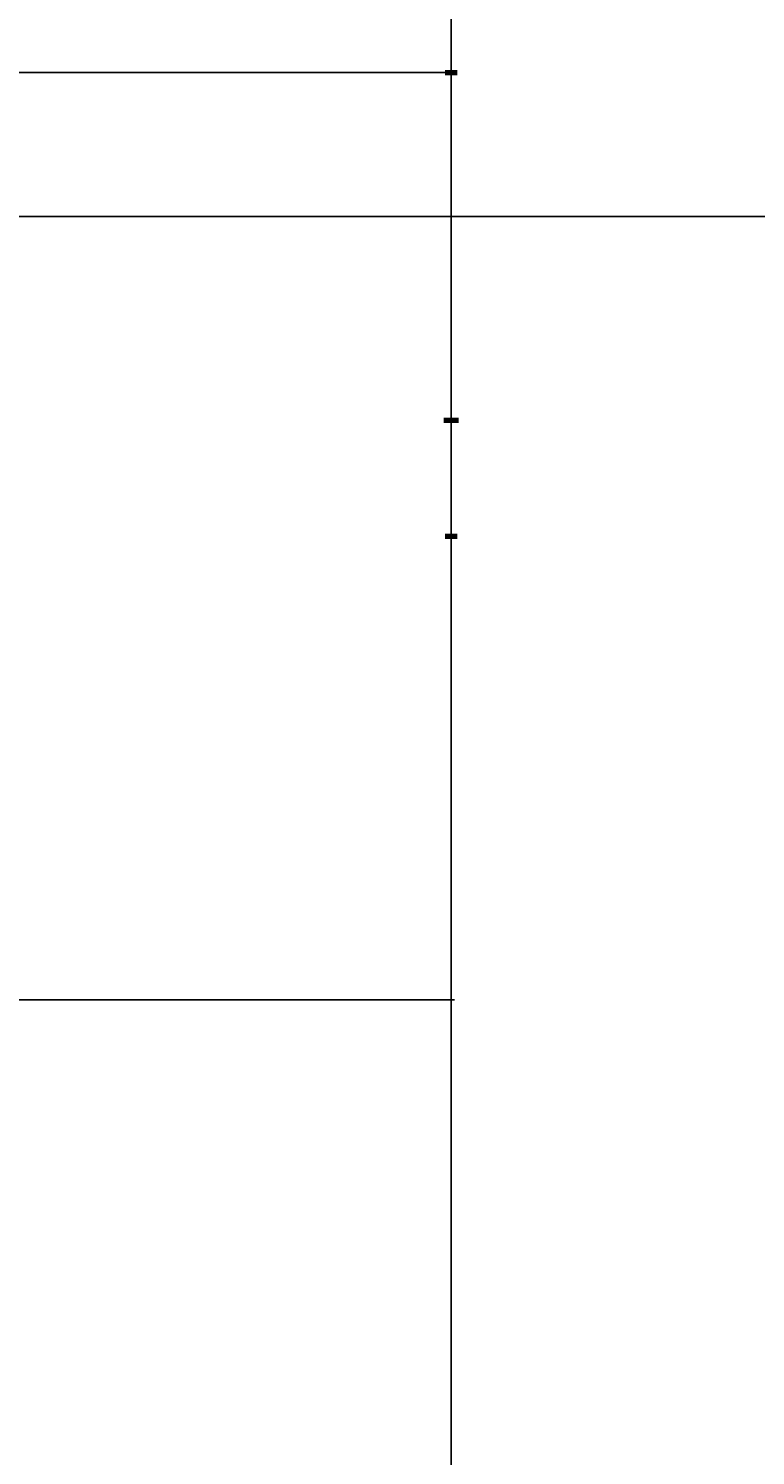
# Model space of a CAD drawing. Units: inches. Extents: x -128 to 854, y -395 to 398.
# Tile 53 of 61: x 368 to 405, y -322 to -248. Entities that reach past the tile are written whole.
import ezdxf

# ---------------------------------------------------------------- set-up
doc = ezdxf.new("R2010")
doc.units = ezdxf.units.IN
doc.header["$MEASUREMENT"] = 0
doc.layers.add('A-ANNO-DIMS', color=2, linetype='Continuous', lineweight=18)
doc.styles.get("Standard").update_dxf_attribs({"font": 'arial.ttf'})
doc.dimstyles.get("Standard").update_dxf_attribs({"dimtxt": 0.18, "dimasz": 0.18, "dimexe": 0.18, "dimexo": 0.0625, "dimgap": 0.09, "dimtad": 0, "dimtih": 1, "dimtoh": 1, "dimdec": 1, "dimzin": 0, "dimdsep": 46, "dimlunit": 4, "dimtxsty": 'Standard', "dimcen": 0.09, "dimclrd": 1, "dimclre": 2, "dimclrt": 6, "dimadec": 0, "dimazin": 0, "dimtfac": 1, "dimtdec": 1, "dimtofl": 0, "dimtmove": 0, "dimatfit": 3, "dimfxl": 1, "dimtfill": 2, "dimtfillclr": 3, "dimtolj": 1, "dimtzin": 0, "dimarcsym": 0})

# ---------------------------------------------------------------- blocks, each defined once
blk = doc.blocks.new('*D120')
at = {"layer": 'A-ANNO-DIMS', "color": 2, "lineweight": -2, "transparency": 16777216}
for p, q in [((317.902, -178.019), (389.719, -178.019)), ((337.902, -358.019), (389.719, -358.019))]:
    blk.add_line(p, q, dxfattribs=at)
at = {"layer": 'A-ANNO-DIMS', "color": 1, "lineweight": -2, "transparency": 16777216}
for p, q in [((389.539, -178.199), (389.539, -267.837)), ((389.539, -357.839), (389.539, -268.201))]:
    blk.add_line(p, q, dxfattribs=at)
at = {"layer": 'A-ANNO-DIMS', "color": 1, "transparency": 16777216}
for points in [[(389.509, -178.199), (389.569, -178.199), (389.539, -178.019)], [(389.509, -357.839), (389.569, -357.839), (389.539, -358.019)]]:
    blk.add_solid(points, dxfattribs=at)
at = {"layer": 'Defpoints', "color": 0, "transparency": 16777216}
for p in [(317.839, -178.019), (337.839, -358.019), (389.539, -358.019)]:
    blk.add_point(p, dxfattribs=at)
at = {"layer": 'A-ANNO-DIMS', "color": 6, "transparency": 16777216, "insert": (389.539, -268.019), "char_height": 0.18, "attachment_point": 5, "bg_fill": 1, "box_fill_scale": 1.25, "bg_fill_color": 3, "bg_fill_transparency": 0}
blk.add_mtext('\\A1;15\'-0"', dxfattribs=at)
blk = doc.blocks.new('*D127')
at = {"layer": 'A-ANNO-DIMS', "color": 2, "lineweight": -2, "transparency": 16777216}
for p, q in [((260.902, -202.019), (389.719, -202.019)), ((317.902, -298.019), (389.719, -298.019))]:
    blk.add_line(p, q, dxfattribs=at)
at = {"layer": 'A-ANNO-DIMS', "color": 1, "lineweight": -2, "transparency": 16777216}
for p, q in [((389.539, -202.199), (389.539, -249.837)), ((389.539, -297.839), (389.539, -250.201))]:
    blk.add_line(p, q, dxfattribs=at)
at = {"layer": 'A-ANNO-DIMS', "color": 1, "transparency": 16777216}
for points in [[(389.509, -202.199), (389.569, -202.199), (389.539, -202.019)], [(389.509, -297.839), (389.569, -297.839), (389.539, -298.019)]]:
    blk.add_solid(points, dxfattribs=at)
at = {"layer": 'Defpoints', "color": 0, "transparency": 16777216}
for p in [(260.839, -202.019), (389.539, -202.019), (317.839, -298.019)]:
    blk.add_point(p, dxfattribs=at)
at = {"layer": 'A-ANNO-DIMS', "color": 6, "transparency": 16777216, "insert": (389.539, -250.019), "char_height": 0.18, "attachment_point": 5, "bg_fill": 1, "box_fill_scale": 1.25, "bg_fill_color": 3, "bg_fill_transparency": 0}
blk.add_mtext('\\A1;8\'-0"', dxfattribs=at)
blk = doc.blocks.new('*D132')
at = {"layer": 'A-ANNO-DIMS', "color": 2, "lineweight": -2, "transparency": 16777216}
for p, q in [((198.902, -250.019), (389.719, -250.019)), ((160.902, -298.019), (389.719, -298.019))]:
    blk.add_line(p, q, dxfattribs=at)
at = {"layer": 'A-ANNO-DIMS', "color": 1, "lineweight": -2, "transparency": 16777216}
for p, q in [((389.539, -250.199), (389.539, -273.837)), ((389.539, -297.839), (389.539, -274.201))]:
    blk.add_line(p, q, dxfattribs=at)
at = {"layer": 'A-ANNO-DIMS', "color": 1, "transparency": 16777216}
for points in [[(389.509, -250.199), (389.569, -250.199), (389.539, -250.019)], [(389.509, -297.839), (389.569, -297.839), (389.539, -298.019)]]:
    blk.add_solid(points, dxfattribs=at)
at = {"layer": 'Defpoints', "color": 0, "transparency": 16777216}
for p in [(198.839, -250.019), (389.539, -250.019), (160.839, -298.019)]:
    blk.add_point(p, dxfattribs=at)
at = {"layer": 'A-ANNO-DIMS', "color": 6, "transparency": 16777216, "insert": (389.539, -274.019), "char_height": 0.18, "attachment_point": 5, "bg_fill": 1, "box_fill_scale": 1.25, "bg_fill_color": 3, "bg_fill_transparency": 0}
blk.add_mtext('\\A1;4\'-0"', dxfattribs=at)
blk = doc.blocks.new('*D134')
at = {"layer": 'A-ANNO-DIMS', "color": 2, "lineweight": -2, "transparency": 16777216}
for p, q in [((418.217, -191.476), (346.3, -191.476)), ((418.217, -371.476), (346.3, -371.476))]:
    blk.add_line(p, q, dxfattribs=at)
at = {"layer": 'A-ANNO-DIMS', "color": 1, "lineweight": -2, "transparency": 16777216}
for p, q in [((346.48, -191.656), (346.48, -281.295)), ((346.48, -371.296), (346.48, -281.658))]:
    blk.add_line(p, q, dxfattribs=at)
at = {"layer": 'A-ANNO-DIMS', "color": 1, "transparency": 16777216}
for points in [[(346.45, -191.656), (346.51, -191.656), (346.48, -191.476)], [(346.45, -371.296), (346.51, -371.296), (346.48, -371.476)]]:
    blk.add_solid(points, dxfattribs=at)
at = {"layer": 'Defpoints', "color": 0, "transparency": 16777216}
for p in [(346.48, -191.476), (418.28, -191.476), (418.28, -371.476)]:
    blk.add_point(p, dxfattribs=at)
at = {"layer": 'A-ANNO-DIMS', "color": 6, "transparency": 16777216, "insert": (346.48, -281.476), "char_height": 0.18, "attachment_point": 5, "bg_fill": 1, "box_fill_scale": 1.25, "bg_fill_color": 3, "bg_fill_transparency": 0}
blk.add_mtext('\\A1;15\'-0"', dxfattribs=at)
blk = doc.blocks.new('*D140')
at = {"layer": 'A-ANNO-DIMS', "color": 2, "lineweight": -2, "transparency": 16777216}
for p, q in [((551.245, -257.476), (346.3, -257.476)), ((551.245, -353.476), (346.3, -353.476))]:
    blk.add_line(p, q, dxfattribs=at)
at = {"layer": 'A-ANNO-DIMS', "color": 1, "lineweight": -2, "transparency": 16777216}
for p, q in [((346.48, -257.656), (346.48, -305.295)), ((346.48, -353.296), (346.48, -305.658))]:
    blk.add_line(p, q, dxfattribs=at)
at = {"layer": 'A-ANNO-DIMS', "color": 1, "transparency": 16777216}
for points in [[(346.45, -257.656), (346.51, -257.656), (346.48, -257.476)], [(346.45, -353.296), (346.51, -353.296), (346.48, -353.476)]]:
    blk.add_solid(points, dxfattribs=at)
at = {"layer": 'Defpoints', "color": 0, "transparency": 16777216}
for p in [(346.48, -257.476), (551.307, -257.476), (551.307, -353.476)]:
    blk.add_point(p, dxfattribs=at)
at = {"layer": 'A-ANNO-DIMS', "color": 6, "transparency": 16777216, "insert": (346.48, -305.476), "char_height": 0.18, "attachment_point": 5, "bg_fill": 1, "box_fill_scale": 1.25, "bg_fill_color": 3, "bg_fill_transparency": 0}
blk.add_mtext('\\A1;8\'-0"', dxfattribs=at)

msp = doc.modelspace()

# ---------------------------------------------------------------- dimensions: what is measured, and where the dimension line sits
at = {"layer": 'A-ANNO-DIMS'}
for base, p1, p2, picture, middle in [((389.539, -358.019), (317.839, -178.019), (337.839, -358.019), '*D120', (389.539, -268.019)), ((346.48, -191.476), (418.28, -371.476), (418.28, -191.476), '*D134', (346.48, -281.476)), ((389.539, -202.019), (317.839, -298.019), (260.839, -202.019), '*D127', (389.539, -250.019)), ((389.539, -250.019), (160.839, -298.019), (198.839, -250.019), '*D132', (389.539, -274.019)), ((346.48, -257.476), (551.307, -353.476), (551.307, -257.476), '*D140', (346.48, -305.476))]:
    dim = msp.add_linear_dim(base=base, p1=p1, p2=p2, angle=90, dimstyle='Standard', override={"dimdec": 1, "dimlfac": 1, "dimrnd": 0, "dimzin": 1, "dimdsep": 46, "dimlunit": 4, "dimfrac": 2}, dxfattribs=at)
    dim.commit()
    dim.dimension.update_dxf_attribs({"geometry": picture, "text_midpoint": middle})

doc.saveas('drawing.dxf')
